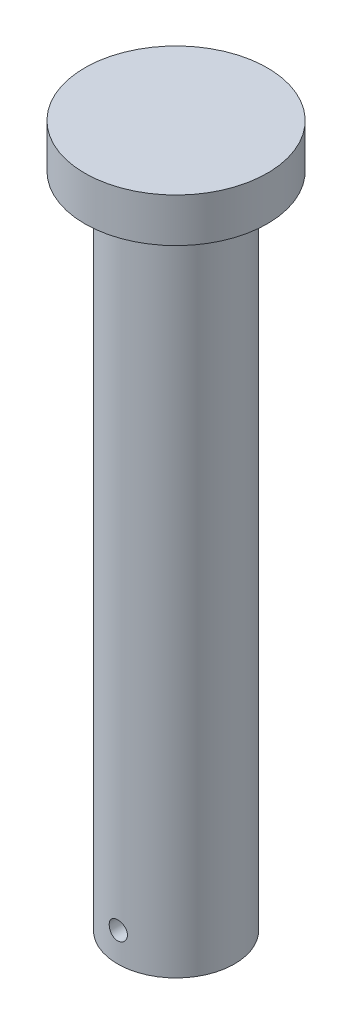
SolidWorks part; units mm, degrees
material "Plain Carbon Steel"
ref_plane "Front Plane" through (0, 0, 0) normal (0, 0, 1) x (1, 0, 0)
ref_plane "Top Plane" through (0, 0, 0) normal (0, 1, 0) x (1, 0, 0)
ref_plane "Right Plane" through (0, 0, 0) normal (1, 0, 0) x (0, 0, -1)
sketch "Head Profile Sketch" plane through (0, 0, 0) normal (0, 1, 0) x (1, 0, 0)
  circle A0 centre (0, 0) radius 25
  dimension "D1" = 50
extrude "Head Ø50x12" add sketch "Head Profile Sketch" along normal blind 12
sketch "Shank Profile Sketch" plane through (0, 0, 0) normal (0, -1, 0) x (1, 0, 0)
  circle A0 centre (0, 0) radius 16
  dimension "D1" = 32
extrude "Shank Ø32x180" add sketch "Shank Profile Sketch" along normal blind 180
sketch "Cross Hole Sketch" plane through (0, 0, 0) normal (0, 0, 1) x (1, 0, 0)
  line L0 (-16, -180) -> (16, -180) construction
  circle A0 centre (0, -172) radius 2.5
  dimension "D1" = 5
  dimension "D2" = 8
  dimension "D3" = 16
extrude "Cross Hole Ø5" cut sketch "Cross Hole Sketch" against normal mid plane 180
